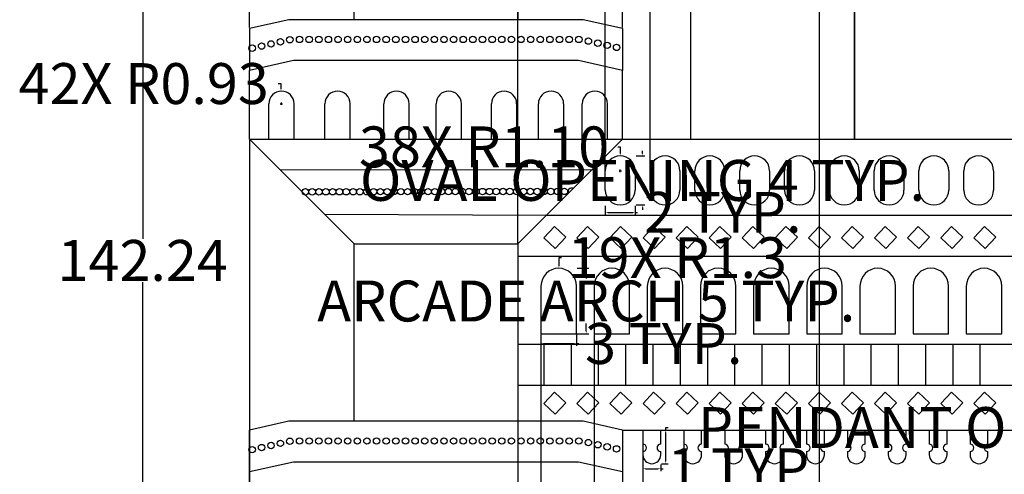
# Model space of a CAD drawing. Units: inches. Extents: x 168 to 318, y 152 to 314.
# Tile 4 of 7: x 168 to 240, y 218 to 251. Entities that reach past the tile are written whole.
import ezdxf

# ---------------------------------------------------------------- set-up
doc = ezdxf.new("R2010")
doc.units = ezdxf.units.IN
doc.header["$MEASUREMENT"] = 0
doc.layers.add('A-ANNO-DIMS', color=2, linetype='Continuous', lineweight=18)
doc.layers.add('A-ELEV', color=7, linetype='Continuous', lineweight=25)
doc.styles.get("Standard").update_dxf_attribs({"font": 'arial.ttf'})
doc.dimstyles.get("Standard").update_dxf_attribs({"dimtxt": 3, "dimasz": 0.18, "dimexe": 0.18, "dimexo": 0.0625, "dimgap": 0.09, "dimtad": 0, "dimtih": 1, "dimtoh": 1, "dimdec": 1, "dimzin": 0, "dimdsep": 46, "dimlunit": 3, "dimtxsty": 'Standard', "dimcen": 0.09, "dimadec": 0, "dimazin": 0, "dimtfac": 1, "dimtdec": 1, "dimtofl": 0, "dimtmove": 0, "dimatfit": 3, "dimfxl": 1, "dimtolj": 1, "dimtzin": 0, "dimarcsym": 0})

# ---------------------------------------------------------------- blocks, each defined once
blk = doc.blocks.new('ORN-PENDANT')
for p, q in [((0, 2.469), (0, 1.437)), ((1.31, 1.437), (1.31, 2.469)), ((0, 0.893), (0, 0.655)), ((1.31, 0.655), (1.31, 0.893))]:
    blk.add_line(p, q)
for centre, radius, start, end in [((0, 1.165), 0.272, 270, 90), ((1.31, 1.165), 0.272, 90, 270), ((0.655, 0.655), 0.655, 180, 0)]:
    blk.add_arc(centre, radius, start, end)
blk = doc.blocks.new('ARCH-BALCONY-SM')
for p, q in [((0, 0), (0, 2.603)), ((1.853, 0), (1.853, 2.603))]:
    blk.add_line(p, q)
blk.add_arc((0.926, 2.603), 0.926, 0, 180)
blk = doc.blocks.new('ARCH-ARCADE')
for p, q in [((0, 3.498), (0, 0)), ((2.6, 0), (2.6, 3.498)), ((0, 0), (2.6, 0))]:
    blk.add_line(p, q)
blk.add_arc((1.3, 3.498), 1.3, 0, 180)
blk = doc.blocks.new('OPENING-OVAL')
for p, q in [((0, 1.096), (0, 2.508)), ((2.191, 2.508), (2.191, 1.096))]:
    blk.add_line(p, q)
for centre, start, end in [((1.095, 2.508), 0, 180), ((1.095, 1.096), 180, 0)]:
    blk.add_arc(centre, 1.095, start, end)
blk = doc.blocks.new('MINARET-UPPER-STAGE')
for p, q in [((0, 24.84), (0, 22.342)), ((22.231, 24.84), (22.231, 22.343)), ((0, 18.24), (0, 22.342)), ((22.231, 18.24), (22.231, 22.342)), ((6.24, 12), (0, 18.24)), ((0, 18.24), (22.231, 18.24)), ((15.991, 12), (22.231, 18.24)), ((5.072, 0), (5.072, 12)), ((6.24, 12), (5.072, 12)), ((6.24, 12), (15.991, 12)), ((6.24, 12), (15.991, 12)), ((15.991, 12), (17.072, 12)), ((17.072, 12), (17.072, 0))]:
    blk.add_line(p, q)
for points in [[(22.231, 24.84), (19.881, 25.365), (2.344, 25.365), (0, 24.84)], [(22.231, 22.343), (19.612, 22.928), (2.613, 22.928), (0, 22.342)]]:
    blk.add_lwpolyline(points)
blk = doc.blocks.new('*D15')
at = {"layer": 'A-ANNO-DIMS', "color": 0, "lineweight": -2, "ltscale": 0.2, "transparency": 16777216}
for p, q in [((215.254, 220.875), (215.254, 221.055)), ((215.254, 221.055), (215.434, 221.055)), ((214.946, 220.875), (215.434, 220.875)), ((215.254, 218.586), (215.254, 220.695)), ((214.946, 218.406), (215.434, 218.406))]:
    blk.add_line(p, q, dxfattribs=at)
at = {"layer": 'A-ANNO-DIMS', "color": 0, "ltscale": 0.2, "transparency": 16777216}
for points in [[(215.224, 220.695), (215.284, 220.695), (215.254, 220.875)], [(215.224, 218.586), (215.284, 218.586), (215.254, 218.406)]]:
    blk.add_solid(points, dxfattribs=at)
at = {"layer": 'Defpoints', "color": 0, "ltscale": 0.2, "transparency": 16777216}
for p in [(214.883, 220.875), (215.254, 220.875), (214.883, 218.406)]:
    blk.add_point(p, dxfattribs=at)
at = {"layer": 'A-ANNO-DIMS', "color": 0, "ltscale": 0.2, "transparency": 16777216, "insert": (244.753, 221.055), "char_height": 3, "attachment_point": 5}
blk.add_mtext('\\A1;PENDANT ORNAMENT 2 TYP.', dxfattribs=at)
blk = doc.blocks.new('*D16')
at = {"layer": 'A-ANNO-DIMS', "color": 0, "lineweight": -2, "ltscale": 0.2, "transparency": 16777216}
for p, q in [((213.573, 218.343), (213.573, 217.855)), ((214.883, 218.343), (214.883, 217.855)), ((213.753, 218.035), (214.703, 218.035)), ((214.883, 218.035), (215.063, 218.035))]:
    blk.add_line(p, q, dxfattribs=at)
at = {"layer": 'A-ANNO-DIMS', "color": 0, "ltscale": 0.2, "transparency": 16777216}
for points in [[(213.753, 218.065), (213.753, 218.005), (213.573, 218.035)], [(214.703, 218.065), (214.703, 218.005), (214.883, 218.035)]]:
    blk.add_solid(points, dxfattribs=at)
at = {"layer": 'Defpoints', "color": 0, "ltscale": 0.2, "transparency": 16777216}
for p in [(213.573, 218.406), (214.883, 218.406), (214.883, 218.035)]:
    blk.add_point(p, dxfattribs=at)
at = {"layer": 'A-ANNO-DIMS', "color": 0, "ltscale": 0.2, "transparency": 16777216, "insert": (221.148, 218.035), "char_height": 3, "attachment_point": 5}
blk.add_mtext('\\A1;1 TYP.', dxfattribs=at)
blk = doc.blocks.new('*D17')
at = {"layer": 'A-ANNO-DIMS', "color": 0, "lineweight": -2, "ltscale": 0.2, "transparency": 16777216}
for p, q in [((208.761, 232.736), (209.598, 232.736)), ((209.418, 232.556), (209.418, 231.978)), ((209.418, 228.118), (209.418, 228.696)), ((208.761, 227.938), (209.598, 227.938))]:
    blk.add_line(p, q, dxfattribs=at)
at = {"layer": 'A-ANNO-DIMS', "color": 0, "ltscale": 0.2, "transparency": 16777216}
for points in [[(209.388, 232.556), (209.448, 232.556), (209.418, 232.736)], [(209.388, 228.118), (209.448, 228.118), (209.418, 227.938)]]:
    blk.add_solid(points, dxfattribs=at)
at = {"layer": 'Defpoints', "color": 0, "ltscale": 0.2, "transparency": 16777216}
for p in [(208.699, 232.736), (209.418, 232.736), (208.699, 227.938)]:
    blk.add_point(p, dxfattribs=at)
at = {"layer": 'A-ANNO-DIMS', "color": 0, "ltscale": 0.2, "transparency": 16777216, "insert": (209.418, 230.337), "char_height": 3, "attachment_point": 5}
blk.add_mtext('\\A1;ARCADE ARCH 5 TYP.', dxfattribs=at)
blk = doc.blocks.new('*D18')
at = {"layer": 'A-ANNO-DIMS', "color": 0, "lineweight": -2, "ltscale": 0.2, "transparency": 16777216}
for p, q in [((206.099, 227.876), (206.099, 227.038)), ((208.699, 227.876), (208.699, 227.038)), ((206.279, 227.218), (208.519, 227.218)), ((208.699, 227.218), (208.879, 227.218))]:
    blk.add_line(p, q, dxfattribs=at)
at = {"layer": 'A-ANNO-DIMS', "color": 0, "ltscale": 0.2, "transparency": 16777216}
for points in [[(206.279, 227.248), (206.279, 227.188), (206.099, 227.218)], [(208.519, 227.248), (208.519, 227.188), (208.699, 227.218)]]:
    blk.add_solid(points, dxfattribs=at)
at = {"layer": 'Defpoints', "color": 0, "ltscale": 0.2, "transparency": 16777216}
for p in [(206.099, 227.938), (208.699, 227.938), (208.699, 227.218)]:
    blk.add_point(p, dxfattribs=at)
at = {"layer": 'A-ANNO-DIMS', "color": 0, "ltscale": 0.2, "transparency": 16777216, "insert": (215.104, 227.218), "char_height": 3, "attachment_point": 5}
blk.add_mtext('\\A1;3 TYP.', dxfattribs=at)
blk = doc.blocks.new('*D19')
at = {"layer": 'A-ANNO-DIMS', "color": 0, "lineweight": -2, "ltscale": 0.2, "transparency": 16777216}
for p, q in [((213.548, 241.164), (213.548, 241.344)), ((213.07, 240.984), (213.728, 240.984)), ((213.07, 237.381), (213.728, 237.381)), ((213.548, 237.201), (213.548, 237.021))]:
    blk.add_line(p, q, dxfattribs=at)
at = {"layer": 'A-ANNO-DIMS', "color": 0, "ltscale": 0.2, "transparency": 16777216}
for points in [[(213.518, 241.164), (213.578, 241.164), (213.548, 240.984)], [(213.518, 237.201), (213.578, 237.201), (213.548, 237.381)]]:
    blk.add_solid(points, dxfattribs=at)
at = {"layer": 'Defpoints', "color": 0, "ltscale": 0.2, "transparency": 16777216}
for p in [(213.008, 240.984), (213.548, 240.984), (213.008, 237.381)]:
    blk.add_point(p, dxfattribs=at)
at = {"layer": 'A-ANNO-DIMS', "color": 0, "ltscale": 0.2, "transparency": 16777216, "insert": (213.548, 239.183), "char_height": 3, "attachment_point": 5}
blk.add_mtext('\\A1;OVAL OPENING 4 TYP.', dxfattribs=at)
blk = doc.blocks.new('*D20')
at = {"layer": 'A-ANNO-DIMS', "color": 0, "lineweight": -2, "ltscale": 0.2, "transparency": 16777216}
for p, q in [((210.817, 237.319), (210.817, 236.661)), ((213.008, 237.319), (213.008, 236.661)), ((210.997, 236.841), (212.828, 236.841)), ((213.008, 236.841), (213.188, 236.841))]:
    blk.add_line(p, q, dxfattribs=at)
at = {"layer": 'A-ANNO-DIMS', "color": 0, "ltscale": 0.2, "transparency": 16777216}
for points in [[(210.997, 236.871), (210.997, 236.811), (210.817, 236.841)], [(212.828, 236.871), (212.828, 236.811), (213.008, 236.841)]]:
    blk.add_solid(points, dxfattribs=at)
at = {"layer": 'Defpoints', "color": 0, "ltscale": 0.2, "transparency": 16777216}
for p in [(210.817, 237.381), (213.008, 237.381), (213.008, 236.841)]:
    blk.add_point(p, dxfattribs=at)
at = {"layer": 'A-ANNO-DIMS', "color": 0, "ltscale": 0.2, "transparency": 16777216, "insert": (219.439, 236.841), "char_height": 3, "attachment_point": 5}
blk.add_mtext('\\A1;2 TYP.', dxfattribs=at)
blk = doc.blocks.new('*D23')
at = {"layer": 'A-ANNO-DIMS', "color": 0, "lineweight": -2, "ltscale": 0.2, "transparency": 16777216}
for p, q in [((261.882, 214.562), (263.075, 214.562)), ((262.895, 214.382), (262.895, 212.619)), ((262.895, 207.574), (262.895, 209.337)), ((261.882, 207.394), (263.075, 207.394))]:
    blk.add_line(p, q, dxfattribs=at)
at = {"layer": 'A-ANNO-DIMS', "color": 0, "ltscale": 0.2, "transparency": 16777216}
for points in [[(262.865, 214.382), (262.925, 214.382), (262.895, 214.562)], [(262.865, 207.574), (262.925, 207.574), (262.895, 207.394)]]:
    blk.add_solid(points, dxfattribs=at)
at = {"layer": 'Defpoints', "color": 0, "ltscale": 0.2, "transparency": 16777216}
for p in [(261.82, 214.562), (262.895, 214.562), (261.82, 207.394)]:
    blk.add_point(p, dxfattribs=at)
at = {"layer": 'A-ANNO-DIMS', "color": 0, "ltscale": 0.2, "transparency": 16777216, "insert": (262.895, 210.978), "char_height": 3, "attachment_point": 5}
blk.add_mtext('\\A1;CUSPED ARCH PANEL 7 TYP.', dxfattribs=at)
blk = doc.blocks.new('*D29')
at = {"layer": 'A-ANNO-DIMS', "color": 0, "lineweight": -2, "ltscale": 0.2, "transparency": 16777216}
for p, q in [((184.724, 242.139), (184.724, 154.215)), ((299.445, 242.139), (299.445, 154.215)), ((184.904, 154.395), (235.924, 154.395)), ((299.265, 154.395), (248.245, 154.395))]:
    blk.add_line(p, q, dxfattribs=at)
at = {"layer": 'A-ANNO-DIMS', "color": 0, "ltscale": 0.2, "transparency": 16777216}
for points in [[(184.904, 154.425), (184.904, 154.365), (184.724, 154.395)], [(299.265, 154.425), (299.265, 154.365), (299.445, 154.395)]]:
    blk.add_solid(points, dxfattribs=at)
at = {"layer": 'Defpoints', "color": 0, "ltscale": 0.2, "transparency": 16777216}
for p in [(184.724, 242.201), (299.445, 242.201), (299.445, 154.395)]:
    blk.add_point(p, dxfattribs=at)
at = {"layer": 'A-ANNO-DIMS', "color": 0, "ltscale": 0.2, "transparency": 16777216, "insert": (242.084, 154.395), "char_height": 3, "attachment_point": 5}
blk.add_mtext('\\A1;114.72', dxfattribs=at)
blk = doc.blocks.new('*D33')
at = {"layer": 'A-ANNO-DIMS', "color": 0, "lineweight": -2, "ltscale": 0.2, "transparency": 16777216}
for p, q in [((198.342, 304.431), (176.701, 304.431)), ((176.881, 304.251), (176.881, 234.909)), ((176.881, 162.375), (176.881, 231.717)), ((192.342, 162.195), (176.701, 162.195))]:
    blk.add_line(p, q, dxfattribs=at)
at = {"layer": 'A-ANNO-DIMS', "color": 0, "ltscale": 0.2, "transparency": 16777216}
for points in [[(176.851, 304.251), (176.911, 304.251), (176.881, 304.431)], [(176.851, 162.375), (176.911, 162.375), (176.881, 162.195)]]:
    blk.add_solid(points, dxfattribs=at)
at = {"layer": 'Defpoints', "color": 0, "ltscale": 0.2, "transparency": 16777216}
for p in [(176.881, 304.431), (198.404, 304.431), (192.404, 162.195)]:
    blk.add_point(p, dxfattribs=at)
at = {"layer": 'A-ANNO-DIMS', "color": 0, "ltscale": 0.2, "transparency": 16777216, "insert": (176.881, 233.313), "char_height": 3, "attachment_point": 5}
blk.add_mtext('\\A1;142.24', dxfattribs=at)
blk = doc.blocks.new('*D57')
at = {"layer": 'A-ANNO-DIMS', "color": 0, "lineweight": -2, "ltscale": 0.2, "transparency": 16777216}
for p, q in [((226.54, 195.647), (226.54, 312.411)), ((226.72, 312.231), (236.931, 312.231)), ((257.449, 312.231), (247.238, 312.231)), ((257.629, 195.647), (257.629, 312.411))]:
    blk.add_line(p, q, dxfattribs=at)
at = {"layer": 'A-ANNO-DIMS', "color": 0, "ltscale": 0.2, "transparency": 16777216}
for points in [[(226.72, 312.261), (226.72, 312.201), (226.54, 312.231)], [(257.449, 312.261), (257.449, 312.201), (257.629, 312.231)]]:
    blk.add_solid(points, dxfattribs=at)
at = {"layer": 'Defpoints', "color": 0, "ltscale": 0.2, "transparency": 16777216}
for p in [(257.629, 312.231), (226.54, 195.584), (257.629, 195.584)]:
    blk.add_point(p, dxfattribs=at)
at = {"layer": 'A-ANNO-DIMS', "color": 0, "ltscale": 0.2, "transparency": 16777216, "insert": (242.084, 312.231), "char_height": 3, "attachment_point": 5}
blk.add_mtext('\\A1;31.09', dxfattribs=at)
blk = doc.blocks.new('*D66')
at = {"layer": 'A-ANNO-DIMS', "color": 0, "lineweight": -2, "ltscale": 0.2, "transparency": 16777216}
for p, q in [((184.724, 250.387), (184.724, 312.411)), ((184.904, 312.231), (193.228, 312.231)), ((211.904, 312.231), (203.581, 312.231)), ((212.084, 250.387), (212.084, 312.411))]:
    blk.add_line(p, q, dxfattribs=at)
at = {"layer": 'A-ANNO-DIMS', "color": 0, "ltscale": 0.2, "transparency": 16777216}
for points in [[(184.904, 312.261), (184.904, 312.201), (184.724, 312.231)], [(211.904, 312.261), (211.904, 312.201), (212.084, 312.231)]]:
    blk.add_solid(points, dxfattribs=at)
at = {"layer": 'Defpoints', "color": 0, "ltscale": 0.2, "transparency": 16777216}
for p in [(212.084, 312.231), (184.724, 250.324), (212.084, 250.324)]:
    blk.add_point(p, dxfattribs=at)
at = {"layer": 'A-ANNO-DIMS', "color": 0, "ltscale": 0.2, "transparency": 16777216, "insert": (198.404, 312.231), "char_height": 3, "attachment_point": 5}
blk.add_mtext('\\A1;27.36', dxfattribs=at)
blk = doc.blocks.new('*D67')
at = {"layer": 'A-ANNO-DIMS', "color": 0, "lineweight": -2, "ltscale": 0.2, "transparency": 16777216}
for p, q in [((217.088, 242.264), (217.088, 312.411)), ((217.268, 312.231), (221.006, 312.231)), ((228.908, 312.231), (225.17, 312.231)), ((229.088, 242.264), (229.088, 312.411))]:
    blk.add_line(p, q, dxfattribs=at)
at = {"layer": 'A-ANNO-DIMS', "color": 0, "ltscale": 0.2, "transparency": 16777216}
for points in [[(217.268, 312.261), (217.268, 312.201), (217.088, 312.231)], [(228.908, 312.261), (228.908, 312.201), (229.088, 312.231)]]:
    blk.add_solid(points, dxfattribs=at)
at = {"layer": 'Defpoints', "color": 0, "ltscale": 0.2, "transparency": 16777216}
for p in [(229.088, 312.231), (217.088, 242.201), (229.088, 242.201)]:
    blk.add_point(p, dxfattribs=at)
at = {"layer": 'A-ANNO-DIMS', "color": 0, "ltscale": 0.2, "transparency": 16777216, "insert": (223.088, 312.231), "char_height": 3, "attachment_point": 5}
blk.add_mtext('\\A1;12', dxfattribs=at)
blk = doc.blocks.new('*D82')
at = {"layer": 'A-ANNO-DIMS', "color": 0, "lineweight": -2, "ltscale": 0.2, "transparency": 16777216}
for p, q in [((204.404, 234.584), (204.404, 312.411)), ((204.584, 312.231), (210.637, 312.231)), ((210.817, 238.539), (210.817, 312.411)), ((210.817, 312.231), (210.997, 312.231))]:
    blk.add_line(p, q, dxfattribs=at)
at = {"layer": 'A-ANNO-DIMS', "color": 0, "ltscale": 0.2, "transparency": 16777216}
for points in [[(204.584, 312.261), (204.584, 312.201), (204.404, 312.231)], [(210.637, 312.261), (210.637, 312.201), (210.817, 312.231)]]:
    blk.add_solid(points, dxfattribs=at)
at = {"layer": 'Defpoints', "color": 0, "ltscale": 0.2, "transparency": 16777216}
for p in [(210.817, 312.231), (210.817, 238.477), (204.404, 234.521)]:
    blk.add_point(p, dxfattribs=at)
at = {"layer": 'A-ANNO-DIMS', "color": 0, "ltscale": 0.2, "transparency": 16777216, "insert": (216.141, 312.231), "char_height": 3, "attachment_point": 5}
blk.add_mtext('\\A1;6.412', dxfattribs=at)
blk = doc.blocks.new('*D83')
at = {"layer": 'A-ANNO-DIMS', "color": 0, "lineweight": -2, "ltscale": 0.2, "transparency": 16777216}
for p, q in [((210.817, 238.539), (210.817, 312.411)), ((210.997, 312.231), (213.923, 312.231)), ((214.103, 238.539), (214.103, 312.411)), ((214.103, 312.231), (214.283, 312.231))]:
    blk.add_line(p, q, dxfattribs=at)
at = {"layer": 'A-ANNO-DIMS', "color": 0, "ltscale": 0.2, "transparency": 16777216}
for points in [[(210.997, 312.261), (210.997, 312.201), (210.817, 312.231)], [(213.923, 312.261), (213.923, 312.201), (214.103, 312.231)]]:
    blk.add_solid(points, dxfattribs=at)
at = {"layer": 'Defpoints', "color": 0, "ltscale": 0.2, "transparency": 16777216}
for p in [(214.103, 312.231), (210.817, 238.477), (214.103, 238.477)]:
    blk.add_point(p, dxfattribs=at)
at = {"layer": 'A-ANNO-DIMS', "color": 0, "ltscale": 0.2, "transparency": 16777216, "insert": (218.272, 312.231), "char_height": 3, "attachment_point": 5}
blk.add_mtext('\\A1;3.29', dxfattribs=at)
blk = doc.blocks.new('*D84')
at = {"layer": 'A-ANNO-DIMS', "color": 0, "lineweight": -2, "ltscale": 0.2, "transparency": 16777216}
for p, q in [((206.099, 227.876), (206.099, 154.215)), ((204.404, 227.113), (204.404, 154.215)), ((204.584, 154.395), (205.919, 154.395)), ((206.099, 154.395), (206.279, 154.395))]:
    blk.add_line(p, q, dxfattribs=at)
at = {"layer": 'A-ANNO-DIMS', "color": 0, "ltscale": 0.2, "transparency": 16777216}
for points in [[(204.584, 154.425), (204.584, 154.365), (204.404, 154.395)], [(205.919, 154.425), (205.919, 154.365), (206.099, 154.395)]]:
    blk.add_solid(points, dxfattribs=at)
at = {"layer": 'Defpoints', "color": 0, "ltscale": 0.2, "transparency": 16777216}
for p in [(206.099, 227.938), (204.404, 227.175), (206.099, 154.395)]:
    blk.add_point(p, dxfattribs=at)
at = {"layer": 'A-ANNO-DIMS', "color": 0, "ltscale": 0.2, "transparency": 16777216, "insert": (211.283, 154.395), "char_height": 3, "attachment_point": 5}
blk.add_mtext('\\A1;1.694', dxfattribs=at)
blk = doc.blocks.new('*D85')
at = {"layer": 'A-ANNO-DIMS', "color": 0, "lineweight": -2, "ltscale": 0.2, "transparency": 16777216}
for p, q in [((206.099, 227.876), (206.099, 154.215)), ((209.999, 227.876), (209.999, 154.215)), ((206.279, 154.395), (209.819, 154.395)), ((209.999, 154.395), (210.179, 154.395))]:
    blk.add_line(p, q, dxfattribs=at)
at = {"layer": 'A-ANNO-DIMS', "color": 0, "ltscale": 0.2, "transparency": 16777216}
for points in [[(206.279, 154.425), (206.279, 154.365), (206.099, 154.395)], [(209.819, 154.425), (209.819, 154.365), (209.999, 154.395)]]:
    blk.add_solid(points, dxfattribs=at)
at = {"layer": 'Defpoints', "color": 0, "ltscale": 0.2, "transparency": 16777216}
for p in [(206.099, 227.938), (209.999, 227.938), (209.999, 154.395)]:
    blk.add_point(p, dxfattribs=at)
at = {"layer": 'A-ANNO-DIMS', "color": 0, "ltscale": 0.2, "transparency": 16777216, "insert": (213.002, 154.395), "char_height": 3, "attachment_point": 5}
blk.add_mtext('\\A1;3.9', dxfattribs=at)
blk = doc.blocks.new('*D86')
at = {"layer": 'A-ANNO-DIMS', "color": 0, "lineweight": -2, "ltscale": 0.2, "transparency": 16777216}
for p, q in [((212.084, 220.813), (212.084, 154.215)), ((213.573, 220.813), (213.573, 154.215)), ((212.264, 154.395), (213.393, 154.395)), ((213.573, 154.395), (213.753, 154.395))]:
    blk.add_line(p, q, dxfattribs=at)
at = {"layer": 'A-ANNO-DIMS', "color": 0, "ltscale": 0.2, "transparency": 16777216}
for points in [[(212.264, 154.425), (212.264, 154.365), (212.084, 154.395)], [(213.393, 154.425), (213.393, 154.365), (213.573, 154.395)]]:
    blk.add_solid(points, dxfattribs=at)
at = {"layer": 'Defpoints', "color": 0, "ltscale": 0.2, "transparency": 16777216}
for p in [(212.084, 220.875), (213.573, 220.875), (213.573, 154.395)]:
    blk.add_point(p, dxfattribs=at)
at = {"layer": 'A-ANNO-DIMS', "color": 0, "ltscale": 0.2, "transparency": 16777216, "insert": (217.601, 154.395), "char_height": 3, "attachment_point": 5}
blk.add_mtext('\\A1;1.49', dxfattribs=at)
blk = doc.blocks.new('*D87')
at = {"layer": 'A-ANNO-DIMS', "color": 0, "lineweight": -2, "ltscale": 0.2, "transparency": 16777216}
for p, q in [((213.573, 220.813), (213.573, 154.215)), ((216.573, 220.813), (216.573, 154.215)), ((213.753, 154.395), (214.001, 154.395)), ((216.393, 154.395), (216.145, 154.395))]:
    blk.add_line(p, q, dxfattribs=at)
at = {"layer": 'A-ANNO-DIMS', "color": 0, "ltscale": 0.2, "transparency": 16777216}
for points in [[(213.753, 154.425), (213.753, 154.365), (213.573, 154.395)], [(216.393, 154.425), (216.393, 154.365), (216.573, 154.395)]]:
    blk.add_solid(points, dxfattribs=at)
at = {"layer": 'Defpoints', "color": 0, "ltscale": 0.2, "transparency": 16777216}
for p in [(213.573, 220.875), (216.573, 220.875), (216.573, 154.395)]:
    blk.add_point(p, dxfattribs=at)
at = {"layer": 'A-ANNO-DIMS', "color": 0, "ltscale": 0.2, "transparency": 16777216, "insert": (215.073, 154.395), "char_height": 3, "attachment_point": 5}
blk.add_mtext('\\A1;3', dxfattribs=at)
blk = doc.blocks.new('*D102')
at = {"layer": 'A-ANNO-DIMS', "color": 0, "lineweight": -2, "ltscale": 0.2, "transparency": 16777216}
for p, q in [((214.629, 214.372), (214.809, 214.372)), ((214.719, 214.282), (214.719, 214.462)), ((216.243, 214.27), (215.851, 214.296))]:
    blk.add_line(p, q, dxfattribs=at)
at = {"layer": 'A-ANNO-DIMS', "color": 0, "ltscale": 0.2, "transparency": 16777216}
blk.add_solid([(215.853, 214.326), (215.849, 214.266), (215.671, 214.308)], dxfattribs=at)
at = {"layer": 'Defpoints', "color": 0, "ltscale": 0.2, "transparency": 16777216}
for p in [(213.766, 214.435), (215.671, 214.308)]:
    blk.add_point(p, dxfattribs=at)
at = {"layer": 'A-ANNO-DIMS', "color": 0, "ltscale": 0.2, "transparency": 16777216, "insert": (224.717, 214.27), "char_height": 3, "attachment_point": 5}
blk.add_mtext('\\A1;8X ∅1.91', dxfattribs=at)
blk = doc.blocks.new('*D103')
at = {"layer": 'A-ANNO-DIMS', "color": 0, "lineweight": -2, "ltscale": 0.2, "transparency": 16777216}
for p, q in [((186.827, 246.285), (187.007, 246.285)), ((187.007, 246.285), (187.021, 245.909)), ((187.06, 244.714), (187.06, 244.894)), ((186.97, 244.804), (187.15, 244.804))]:
    blk.add_line(p, q, dxfattribs=at)
at = {"layer": 'A-ANNO-DIMS', "color": 0, "ltscale": 0.2, "transparency": 16777216}
blk.add_solid([(187.051, 245.91), (186.991, 245.908), (187.027, 245.729)], dxfattribs=at)
at = {"layer": 'Defpoints', "color": 0, "ltscale": 0.2, "transparency": 16777216}
for p in [(187.027, 245.729), (187.06, 244.804)]:
    blk.add_point(p, dxfattribs=at)
at = {"layer": 'A-ANNO-DIMS', "color": 0, "ltscale": 0.2, "transparency": 16777216, "insert": (176.957, 246.285), "char_height": 3, "attachment_point": 5}
blk.add_mtext('\\A1;42X R0.93', dxfattribs=at)
blk = doc.blocks.new('*D104')
at = {"layer": 'A-ANNO-DIMS', "color": 0, "lineweight": -2, "ltscale": 0.2, "transparency": 16777216}
for p, q in [((207.417, 233.516), (207.412, 232.916)), ((207.597, 233.516), (207.417, 233.516)), ((207.309, 231.436), (207.489, 231.436)), ((207.399, 231.346), (207.399, 231.526))]:
    blk.add_line(p, q, dxfattribs=at)
at = {"layer": 'A-ANNO-DIMS', "color": 0, "ltscale": 0.2, "transparency": 16777216}
blk.add_solid([(207.382, 232.916), (207.442, 232.916), (207.41, 232.736)], dxfattribs=at)
at = {"layer": 'Defpoints', "color": 0, "ltscale": 0.2, "transparency": 16777216}
for p in [(207.41, 232.736), (207.399, 231.436)]:
    blk.add_point(p, dxfattribs=at)
at = {"layer": 'A-ANNO-DIMS', "color": 0, "ltscale": 0.2, "transparency": 16777216, "insert": (216.101, 233.516), "char_height": 3, "attachment_point": 5}
blk.add_mtext('\\A1;19X R1.3', dxfattribs=at)
blk = doc.blocks.new('*D105')
at = {"layer": 'A-ANNO-DIMS', "color": 0, "lineweight": -2, "ltscale": 0.2, "transparency": 16777216}
for p, q in [((211.729, 241.641), (211.909, 241.641)), ((211.909, 241.641), (211.91, 241.164)), ((211.822, 239.889), (212.002, 239.889)), ((211.912, 239.799), (211.912, 239.979))]:
    blk.add_line(p, q, dxfattribs=at)
at = {"layer": 'A-ANNO-DIMS', "color": 0, "ltscale": 0.2, "transparency": 16777216}
blk.add_solid([(211.94, 241.164), (211.88, 241.164), (211.91, 240.984)], dxfattribs=at)
at = {"layer": 'Defpoints', "color": 0, "ltscale": 0.2, "transparency": 16777216}
for p in [(211.91, 240.984), (211.912, 239.889)]:
    blk.add_point(p, dxfattribs=at)
at = {"layer": 'A-ANNO-DIMS', "color": 0, "ltscale": 0.2, "transparency": 16777216, "insert": (201.924, 241.641), "char_height": 3, "attachment_point": 5}
blk.add_mtext('\\A1;38X R1.10', dxfattribs=at)

msp = doc.modelspace()

# ---------------------------------------------------------------- linework, layer by layer
at = {"layer": 'A-ELEV'}
for p, q in [((184.7244, 250.3243), (184.7244, 247.25)), ((212.0845, 250.3243), (212.0845, 247.2504)), ((184.7244, 242.2013), (184.7244, 247.25)), ((212.0845, 242.2013), (212.0845, 247.25)), ((192.4044, 234.5213), (184.7244, 242.2013)), ((184.7244, 242.2013), (212.0845, 242.2013)), ((204.4044, 234.5213), (212.0845, 242.2013)), ((212.0845, 242.2013), (272.0845, 242.2013)), ((186.9522, 239.9735), (209.8404, 239.9573)), ((190.2158, 236.7099), (206.511, 236.6279)), ((206.511, 236.6279), (277.6579, 236.6279)), ((192.4044, 221.5213), (192.4044, 234.5213)), ((192.4044, 234.5213), (204.4044, 234.5213)), ((204.4044, 234.5213), (204.4044, 221.5213)), ((204.4044, 233.6213), (279.7645, 233.6213)), ((204.4044, 227.1751), (279.7645, 227.1751)), ((206.3013, 227.1751), (206.3013, 224.1751)), ((208.3013, 227.1751), (208.3013, 224.1751)), ((210.3013, 227.1751), (210.3013, 224.1751)), ((212.3013, 227.1751), (212.3013, 224.1751)), ((214.3013, 227.1751), (214.3013, 224.1751)), ((216.3013, 227.1751), (216.3013, 224.1751)), ((218.3013, 227.1751), (218.3013, 224.1751)), ((220.3013, 227.1751), (220.3013, 224.1751)), ((222.3013, 227.1751), (222.3013, 224.1751)), ((224.3013, 227.1751), (224.3013, 224.1751)), ((226.3013, 227.1751), (226.3013, 224.1751)), ((228.3013, 227.1751), (228.3013, 224.1751)), ((230.3013, 227.1751), (230.3013, 224.1751)), ((232.3013, 227.1751), (232.3013, 224.1751)), ((234.3013, 227.1751), (234.3013, 224.1751)), ((236.3013, 227.1751), (236.3013, 224.1751)), ((238.3013, 227.1751), (238.3013, 224.1751)), ((204.4044, 224.1751), (279.7645, 224.1751)), ((184.7244, 205.8755), (184.7244, 220.8755)), ((212.0845, 220.8755), (212.0845, 205.8755)), ((212.0845, 220.8755), (272.0845, 220.8755))]:
    msp.add_line(p, q, dxfattribs=at)
for points in [[(212.0845, 250.3243), (209.193, 250.9701), (187.6087, 250.9701), (184.7244, 250.3243)], [(212.0845, 247.2504), (208.862, 247.9701), (187.9405, 247.9701), (184.7244, 247.25)], [(212.0845, 220.8755), (209.193, 221.5213), (187.6087, 221.5213), (184.7244, 220.8755)], [(212.0845, 217.8016), (208.862, 218.5213), (187.9405, 218.5213), (184.7244, 217.8012)]]:
    msp.add_lwpolyline(points, dxfattribs=at)
for points in [[(207.9204, 235.0162), (207.0852, 235.7986), (206.3029, 234.9634), (207.1381, 234.1811)], [(210.3467, 235.0162), (209.5115, 235.7986), (208.7292, 234.9634), (209.5643, 234.1811)], [(212.7729, 235.0162), (211.9378, 235.7986), (211.1554, 234.9634), (211.9906, 234.1811)], [(215.1992, 235.0162), (214.364, 235.7986), (213.5817, 234.9634), (214.4168, 234.1811)], [(217.6254, 235.0162), (216.7903, 235.7986), (216.0079, 234.9634), (216.8431, 234.1811)], [(220.0517, 235.0162), (219.2165, 235.7986), (218.4342, 234.9634), (219.2694, 234.1811)], [(222.478, 235.0162), (221.6428, 235.7986), (220.8605, 234.9634), (221.6956, 234.1811)], [(224.9042, 235.0162), (224.0691, 235.7986), (223.2867, 234.9634), (224.1219, 234.1811)], [(227.3305, 235.0162), (226.4953, 235.7986), (225.713, 234.9634), (226.5482, 234.1811)], [(229.7568, 235.0162), (228.9216, 235.7986), (228.1392, 234.9634), (228.9744, 234.1811)], [(232.183, 235.0162), (231.3478, 235.7986), (230.5655, 234.9634), (231.4007, 234.1811)], [(234.6093, 235.0162), (233.7741, 235.7986), (232.9918, 234.9634), (233.8269, 234.1811)], [(237.0355, 235.0162), (236.2004, 235.7986), (235.418, 234.9634), (236.2532, 234.1811)], [(239.4618, 235.0162), (238.6266, 235.7986), (237.8443, 234.9634), (238.6795, 234.1811)], [(207.9204, 222.8812), (207.0852, 223.6635), (206.3029, 222.8284), (207.1381, 222.046)], [(210.3467, 222.8812), (209.5115, 223.6635), (208.7292, 222.8284), (209.5643, 222.046)], [(212.7729, 222.8812), (211.9378, 223.6635), (211.1554, 222.8284), (211.9906, 222.046)], [(215.1992, 222.8812), (214.364, 223.6635), (213.5817, 222.8284), (214.4168, 222.046)], [(217.6254, 222.8812), (216.7903, 223.6635), (216.0079, 222.8284), (216.8431, 222.046)], [(220.0517, 222.8812), (219.2165, 223.6635), (218.4342, 222.8284), (219.2694, 222.046)], [(222.478, 222.8812), (221.6428, 223.6635), (220.8605, 222.8284), (221.6956, 222.046)], [(224.9042, 222.8812), (224.0691, 223.6635), (223.2867, 222.8284), (224.1219, 222.046)], [(227.3305, 222.8812), (226.4953, 223.6635), (225.713, 222.8284), (226.5482, 222.046)], [(229.7568, 222.8812), (228.9216, 223.6635), (228.1392, 222.8284), (228.9744, 222.046)], [(232.183, 222.8812), (231.3478, 223.6635), (230.5655, 222.8284), (231.4007, 222.046)], [(234.6093, 222.8812), (233.7741, 223.6635), (232.9918, 222.8284), (233.8269, 222.046)], [(237.0355, 222.8812), (236.2004, 223.6635), (235.418, 222.8284), (236.2532, 222.046)], [(239.4618, 222.8812), (238.6266, 223.6635), (237.8443, 222.8284), (238.6795, 222.046)]]:
    msp.add_lwpolyline(points, close=True, dxfattribs=at)
for centre in [(185.6052, 249.0371), (186.2945, 249.1914), (186.9837, 249.3457), (187.673, 249.5001), (188.3883, 249.5215), (189.0947, 249.5215), (189.801, 249.5215), (190.5073, 249.5215), (191.2137, 249.5215), (191.92, 249.5215), (192.6263, 249.5215), (193.3326, 249.5215), (194.039, 249.5215), (194.7453, 249.5215), (195.4516, 249.5215), (196.158, 249.5215), (196.8643, 249.5215), (197.5706, 249.5215), (198.2769, 249.5215), (198.9833, 249.5215), (199.6896, 249.5215), (200.3959, 249.5215), (201.1023, 249.5215), (201.8086, 249.5215), (202.5149, 249.5215), (203.2212, 249.5215), (203.9276, 249.5215), (204.6339, 249.5215), (205.3402, 249.5215), (206.0466, 249.5215), (206.7529, 249.5215), (207.4592, 249.5215), (208.1655, 249.5215), (208.8719, 249.5215), (209.5762, 249.4003), (210.2655, 249.2463), (210.9549, 249.0923), (211.6442, 248.9384), (184.916, 248.8828), (188.8149, 238.3462), (189.3149, 238.347), (189.8149, 238.3477), (190.3149, 238.3484), (190.8149, 238.3491), (191.3149, 238.3498), (191.8149, 238.3505), (192.3149, 238.3513), (192.8149, 238.352), (193.3149, 238.3527), (193.8149, 238.3534), (194.3149, 238.3541), (194.8149, 238.3548), (195.3149, 238.3556), (195.8149, 238.3563), (196.3149, 238.357), (196.8149, 238.3577), (197.3149, 238.3584), (197.8149, 238.3591), (198.3149, 238.3599), (198.8149, 238.3606), (199.3149, 238.3613), (199.8149, 238.362), (200.3149, 238.3627), (200.8149, 238.3634), (201.3149, 238.3642), (201.8149, 238.3649), (202.3149, 238.3656), (202.8149, 238.3663), (203.3149, 238.367), (203.8149, 238.3677), (204.3149, 238.3685), (204.8149, 238.3692), (205.3149, 238.3699), (205.8149, 238.3706), (206.3149, 238.3713), (206.8149, 238.372), (207.3149, 238.3728), (207.8149, 238.3735), (187.673, 220.0513), (188.3883, 220.0727), (189.0947, 220.0727), (189.801, 220.0727), (190.5073, 220.0727), (191.2137, 220.0727), (191.92, 220.0727), (192.6263, 220.0727), (193.3326, 220.0727), (194.039, 220.0727), (194.7453, 220.0727), (195.4516, 220.0727), (196.158, 220.0727), (196.8643, 220.0727), (197.5706, 220.0727), (198.2769, 220.0727), (198.9833, 220.0727), (199.6896, 220.0727), (200.3959, 220.0727), (201.1023, 220.0727), (201.8086, 220.0727), (202.5149, 220.0727), (203.2212, 220.0727), (203.9276, 220.0727), (204.6339, 220.0727), (205.3402, 220.0727), (206.0466, 220.0727), (206.7529, 220.0727), (207.4592, 220.0727), (208.1655, 220.0727), (208.8719, 220.0727), (184.916, 219.434), (185.6052, 219.5883), (186.2945, 219.7426), (186.9837, 219.8969), (209.5762, 219.9515), (210.2655, 219.7975), (210.9549, 219.6435), (211.6442, 219.4896)]:
    msp.add_circle(centre, 0.2354, dxfattribs=at)
msp.add_arc((208.3149, 238.3742), 0.2354, 54.95912, 215.04088, dxfattribs=at)

# ---------------------------------------------------------------- block references
for name, p in [('MINARET-UPPER-STAGE', (187.332, 250.97)), ('MINARET-UPPER-STAGE', (212.0154, 242.2012)), ('ARCH-BALCONY-SM', (186.134, 242.2009)), ('ARCH-BALCONY-SM', (190.2525, 242.2009)), ('ARCH-BALCONY-SM', (194.5757, 242.2009)), ('ARCH-BALCONY-SM', (198.4045, 242.2009)), ('ARCH-BALCONY-SM', (202.4627, 242.2009)), ('ARCH-BALCONY-SM', (205.9096, 242.2009)), ('ARCH-BALCONY-SM', (209.1229, 242.2009)), ('OPENING-OVAL', (210.817, 237.381)), ('OPENING-OVAL', (214.1034, 237.381)), ('OPENING-OVAL', (217.3898, 237.381)), ('OPENING-OVAL', (220.6762, 237.381)), ('OPENING-OVAL', (223.9627, 237.381)), ('OPENING-OVAL', (227.2491, 237.381)), ('OPENING-OVAL', (230.5355, 237.381)), ('OPENING-OVAL', (233.8219, 237.381)), ('OPENING-OVAL', (237.1083, 237.381)), ('ARCH-ARCADE', (206.099, 227.938)), ('ARCH-ARCADE', (209.999, 227.938)), ('ARCH-ARCADE', (213.899, 227.938)), ('ARCH-ARCADE', (217.799, 227.938)), ('ARCH-ARCADE', (221.699, 227.938)), ('ARCH-ARCADE', (225.599, 227.938)), ('ARCH-ARCADE', (229.499, 227.938)), ('ARCH-ARCADE', (233.399, 227.938)), ('ARCH-ARCADE', (237.299, 227.938)), ('ORN-PENDANT', (213.573, 218.406)), ('ORN-PENDANT', (216.573, 218.406)), ('ORN-PENDANT', (219.573, 218.406)), ('ORN-PENDANT', (222.573, 218.406)), ('ORN-PENDANT', (225.573, 218.406)), ('ORN-PENDANT', (228.573, 218.406)), ('ORN-PENDANT', (231.573, 218.406)), ('ORN-PENDANT', (234.573, 218.406)), ('ORN-PENDANT', (237.573, 218.406))]:
    msp.add_blockref(name, p, dxfattribs=at)

# ---------------------------------------------------------------- dimensions: what is measured, and where the dimension line sits
at = {"layer": 'A-ANNO-DIMS', "ltscale": 0.2}
for base, p1, p2, override, picture, middle in [((212.0845, 312.2308), (184.7244, 250.3243), (212.0845, 250.3243), {"dimdec": 2, "dimlfac": 1, "dimrnd": 0, "dimzin": 0, "dimdsep": 46, "dimlunit": 2}, '*D66', (198.4044, 312.2308)), ((210.8168, 312.2308), (204.4044, 234.5213), (210.8168, 238.4767), {"dimdec": 3, "dimlfac": 1, "dimrnd": 0, "dimzin": 0, "dimdsep": 46, "dimlunit": 2}, '*D82', (216.1414, 312.2308)), ((214.1032, 312.2308), (210.8168, 238.4767), (214.1032, 238.4767), {"dimdec": 2, "dimlfac": 1, "dimrnd": 0, "dimzin": 0, "dimdsep": 46, "dimlunit": 2}, '*D83', (218.2716, 312.2308)), ((229.0878, 312.2308), (217.0878, 242.2013), (229.0878, 242.2013), {"dimdec": 0, "dimlfac": 1, "dimrnd": 0, "dimzin": 0, "dimdsep": 46, "dimlunit": 2}, '*D67', (223.0878, 312.2308)), ((257.6286, 312.2308), (226.5403, 195.5844), (257.6286, 195.5844), {"dimdec": 2, "dimlfac": 1, "dimrnd": 0, "dimzin": 0, "dimdsep": 46, "dimlunit": 2}, '*D57', (242.0845, 312.2308)), ((299.4446, 154.3954), (184.7244, 242.2013), (299.4446, 242.2013), {"dimdec": 2, "dimlfac": 1, "dimrnd": 0, "dimzin": 0, "dimdsep": 46, "dimlunit": 2}, '*D29', (242.0845, 154.3954)), ((206.0986, 154.3954), (204.4044, 227.1751), (206.0986, 227.9381), {"dimdec": 3, "dimlfac": 1, "dimrnd": 0, "dimzin": 0, "dimdsep": 46, "dimlunit": 2}, '*D84', (211.283, 154.3954)), ((209.9986, 154.3954), (206.0986, 227.9381), (209.9986, 227.9381), {"dimdec": 1, "dimlfac": 1, "dimrnd": 0, "dimzin": 0, "dimdsep": 46, "dimlunit": 2}, '*D85', (213.0015, 154.3954)), ((213.5729, 154.3954), (212.0845, 220.8755), (213.5729, 220.8755), {"dimdec": 2, "dimlfac": 1, "dimrnd": 0, "dimzin": 0, "dimdsep": 46, "dimlunit": 2}, '*D86', (217.601, 154.3954)), ((216.5729, 154.3954), (213.5729, 220.8755), (216.5729, 220.8755), {"dimdec": 0, "dimlfac": 1, "dimrnd": 0, "dimzin": 0, "dimdsep": 46, "dimlunit": 2}, '*D87', (215.0729, 154.3954))]:
    dim = msp.add_linear_dim(base=base, p1=p1, p2=p2, dimstyle='Standard', override=override, dxfattribs=at)
    dim.commit()
    dim.dimension.update_dxf_attribs({"geometry": picture, "text_midpoint": middle})
dim = msp.add_linear_dim(base=(176.8805, 304.4308), p1=(192.4044, 162.1954), p2=(198.4044, 304.4308), angle=90, dimstyle='Standard', override={"dimdec": 2, "dimlfac": 1, "dimrnd": 0, "dimzin": 0, "dimdsep": 46, "dimlunit": 2}, dxfattribs=at)
dim.commit()
dim.dimension.update_dxf_attribs({"geometry": '*D33', "text_midpoint": (176.8805, 233.3131)})
for center, mpoint, text, override, picture, middle in [((187.0603, 244.8037), (187.0272, 245.7294), '42X <>', {"dimdec": 2, "dimlfac": 1, "dimrnd": 0, "dimzin": 0, "dimdsep": 46, "dimlunit": 2}, '*D103', (176.9566, 246.2849)), ((211.9123, 239.8886), (211.91, 240.9841), '38X <>', {"dimdec": 2, "dimlfac": 1, "dimrnd": 0, "dimzin": 0, "dimdsep": 46, "dimlunit": 2}, '*D105', (201.9245, 241.6414)), ((207.3986, 231.4359), (207.4101, 232.7359), '19X <>', {"dimdec": 1, "dimlfac": 1, "dimrnd": 0, "dimzin": 0, "dimdsep": 46, "dimlunit": 2}, '*D104', (216.1008, 233.5158))]:
    dim = msp.add_radius_dim(center=center, mpoint=mpoint, text=text, dimstyle='Standard', override=override, dxfattribs=at)
    dim.commit()
    dim.dimension.update_dxf_attribs({"geometry": picture, "text_midpoint": middle, "dimtype": 164})
for base, p1, p2, text, picture, middle in [((213.5482, 240.9841), (213.0078, 237.3812), (213.0078, 240.9841), 'OVAL OPENING <> TYP.', '*D19', (213.5482, 239.1826)), ((209.4182, 232.7359), (208.6986, 227.9381), (208.6986, 232.7359), 'ARCADE ARCH <> TYP.', '*D17', (209.4182, 230.337)), ((215.2539, 220.8755), (214.8834, 218.4056), (214.8834, 220.8755), 'PENDANT ORNAMENT <> TYP.', '*D15', (244.7534, 221.0555)), ((262.8949, 214.5622), (261.8196, 207.3935), (261.8196, 214.5622), 'CUSPED ARCH PANEL <> TYP.', '*D23', (262.8949, 210.9778))]:
    dim = msp.add_linear_dim(base=base, p1=p1, p2=p2, angle=90, text=text, dimstyle='Standard', override={"dimdec": 0, "dimrnd": 0, "dimzin": 0, "dimlunit": 2}, dxfattribs=at)
    dim.commit()
    dim.dimension.update_dxf_attribs({"geometry": picture, "text_midpoint": middle})
for base, p1, p2, picture, middle in [((213.0078, 236.8407), (210.8168, 237.3812), (213.0078, 237.3812), '*D20', (219.4394, 236.8407)), ((208.6986, 227.2185), (206.0986, 227.9381), (208.6986, 227.9381), '*D18', (215.1036, 227.2185)), ((214.8834, 218.0352), (213.5729, 218.4056), (214.8834, 218.4056), '*D16', (221.1483, 218.0352))]:
    dim = msp.add_linear_dim(base=base, p1=p1, p2=p2, text='<> TYP.', dimstyle='Standard', override={"dimdec": 0, "dimrnd": 0, "dimzin": 0, "dimlunit": 2}, dxfattribs=at)
    dim.commit()
    dim.dimension.update_dxf_attribs({"geometry": picture, "text_midpoint": middle})
dim = msp.add_diameter_dim_2p(p1=(213.7659, 214.4352), p2=(215.6712, 214.3079), text='8X <>', dimstyle='Standard', override={"dimdec": 2, "dimlfac": 1, "dimrnd": 0, "dimzin": 0, "dimdsep": 46, "dimlunit": 2}, dxfattribs=at)
dim.commit()
dim.dimension.update_dxf_attribs({"geometry": '*D102', "text_midpoint": (216.2428, 214.2697), "dimtype": 163})

doc.saveas('drawing.dxf')
